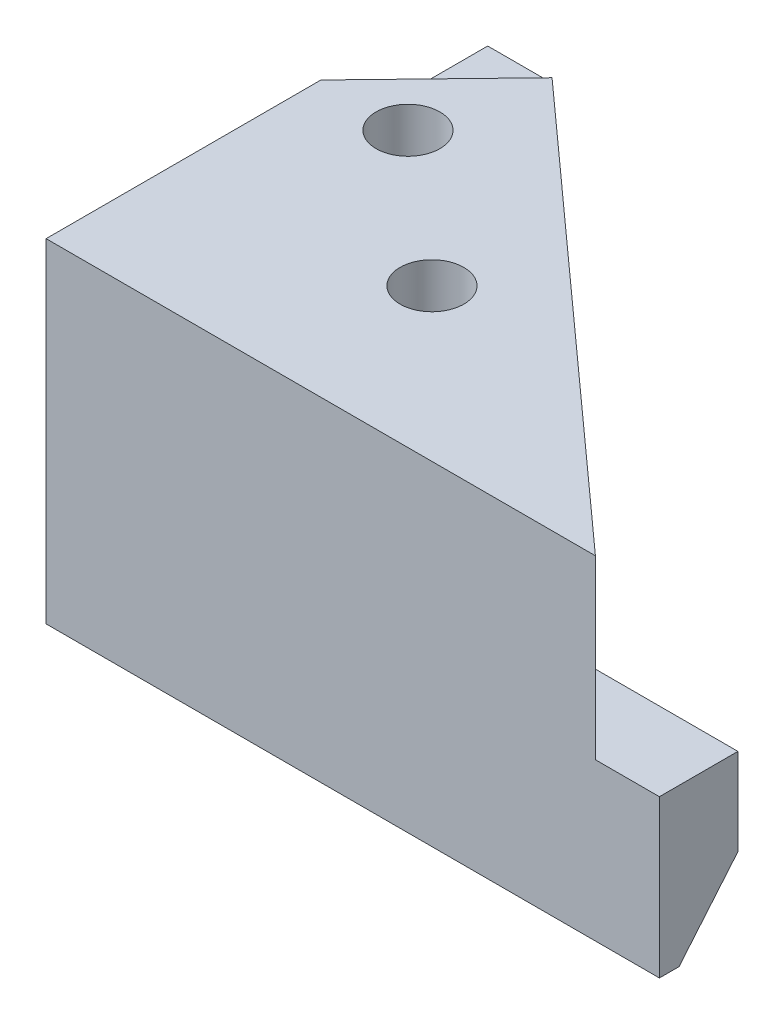
ISO-10303-21;
HEADER;
FILE_DESCRIPTION(('STEP AP214'),'2;1');
FILE_NAME('part.step','',(''),(''),'','','');
FILE_SCHEMA(('AUTOMOTIVE_DESIGN { 1 0 10303 214 1 1 1 1 }'));
ENDSEC;
DATA;
#1=APPLICATION_CONTEXT('core data for automotive mechanical design processes');
#2=APPLICATION_PROTOCOL_DEFINITION('international standard','automotive_design',2000,#1);
#3=PRODUCT_CONTEXT('',#1,'mechanical');
#4=PRODUCT('Part','Part','',(#3));
#5=PRODUCT_RELATED_PRODUCT_CATEGORY('part','',(#4));
#6=PRODUCT_DEFINITION_FORMATION('','',#4);
#7=PRODUCT_DEFINITION_CONTEXT('part definition',#1,'design');
#8=PRODUCT_DEFINITION('design','',#6,#7);
#9=PRODUCT_DEFINITION_SHAPE('','',#8);
#10=(LENGTH_UNIT() NAMED_UNIT(*) SI_UNIT(.MILLI.,.METRE.));
#11=(NAMED_UNIT(*) PLANE_ANGLE_UNIT() SI_UNIT($,.RADIAN.));
#12=(NAMED_UNIT(*) SI_UNIT($,.STERADIAN.) SOLID_ANGLE_UNIT());
#13=UNCERTAINTY_MEASURE_WITH_UNIT(LENGTH_MEASURE(1.E-05),#10,'distance_accuracy_value','');
#14=(GEOMETRIC_REPRESENTATION_CONTEXT(3) GLOBAL_UNCERTAINTY_ASSIGNED_CONTEXT((#13)) GLOBAL_UNIT_ASSIGNED_CONTEXT((#10,
#11,#12)) REPRESENTATION_CONTEXT('',''));
#15=CARTESIAN_POINT('',(0.,0.,0.));
#16=DIRECTION('',(0.,0.,1.));
#17=DIRECTION('',(1.,0.,0.));
#18=AXIS2_PLACEMENT_3D('',#15,#16,#17);
#19=CARTESIAN_POINT('',(0.,36.,0.));
#20=DIRECTION('',(-0.669130606358854,0.,0.743144825477398));
#21=DIRECTION('',(0.743144825477398,0.,0.669130606358854));
#22=AXIS2_PLACEMENT_3D('',#19,#20,#21);
#23=PLANE('',#22);
#24=CARTESIAN_POINT('',(-49.7907033069857,17.,-44.8317506260432));
#25=DIRECTION('',(0.669130606358854,0.,-0.743144825477398));
#26=DIRECTION('',(-0.743144825477398,0.,-0.669130606358854));
#27=AXIS2_PLACEMENT_3D('',#24,#25,#26);
#28=CIRCLE('',#27,6.);
#29=CARTESIAN_POINT('',(-54.2495722598501,17.,-48.8465342641963));
#30=VERTEX_POINT('',#29);
#31=EDGE_CURVE('E312',#30,#30,#28,.T.);
#32=ORIENTED_EDGE('',*,*,#31,.F.);
#33=EDGE_LOOP('',(#32));
#34=FACE_BOUND('',#33,.T.);
#35=DIRECTION('',(0.,-1.,0.));
#36=VECTOR('',#35,1.);
#37=CARTESIAN_POINT('',(-88.8009956275672,266.1095550301,-79.9567756007354));
#38=LINE('',#37,#36);
#39=CARTESIAN_POINT('',(-88.8009956275672,36.,-79.9567756007354));
#40=VERTEX_POINT('',#39);
#41=CARTESIAN_POINT('',(-88.8009956275672,25.,-79.9567756007354));
#42=VERTEX_POINT('',#41);
#43=EDGE_CURVE('E297',#40,#42,#38,.T.);
#44=ORIENTED_EDGE('',*,*,#43,.F.);
#45=DIRECTION('',(-0.743144825477398,0.,-0.669130606358854));
#46=VECTOR('',#45,1.);
#47=CARTESIAN_POINT('',(0.,36.,0.));
#48=LINE('',#47,#46);
#49=CARTESIAN_POINT('',(0.,36.,0.));
#50=VERTEX_POINT('',#49);
#51=EDGE_CURVE('E261',#50,#40,#48,.T.);
#52=ORIENTED_EDGE('',*,*,#51,.F.);
#53=DIRECTION('',(0.,-1.,0.));
#54=VECTOR('',#53,1.);
#55=CARTESIAN_POINT('',(0.,36.,0.));
#56=LINE('',#55,#54);
#57=CARTESIAN_POINT('',(0.,0.,0.));
#58=VERTEX_POINT('',#57);
#59=EDGE_CURVE('E11',#50,#58,#56,.T.);
#60=ORIENTED_EDGE('',*,*,#59,.T.);
#61=DIRECTION('',(-0.743144825477398,0.,-0.669130606358854));
#62=VECTOR('',#61,1.);
#63=CARTESIAN_POINT('',(0.,0.,0.));
#64=LINE('',#63,#62);
#65=CARTESIAN_POINT('',(-17.7698002372673,0.,-16.));
#66=VERTEX_POINT('',#65);
#67=EDGE_CURVE('E262',#58,#66,#64,.T.);
#68=ORIENTED_EDGE('',*,*,#67,.T.);
#69=CARTESIAN_POINT('',(-99.9551263346285,0.,-90.));
#70=VERTEX_POINT('',#69);
#71=EDGE_CURVE('E267',#66,#70,#64,.T.);
#72=ORIENTED_EDGE('',*,*,#71,.T.);
#73=DIRECTION('',(0.,-1.,0.));
#74=VECTOR('',#73,1.);
#75=CARTESIAN_POINT('',(-99.9551263346285,36.,-90.));
#76=LINE('',#75,#74);
#77=CARTESIAN_POINT('',(-99.9551263346285,25.,-90.));
#78=VERTEX_POINT('',#77);
#79=EDGE_CURVE('E47',#78,#70,#76,.T.);
#80=ORIENTED_EDGE('',*,*,#79,.F.);
#81=DIRECTION('',(-0.743144825477398,0.,-0.669130606358854));
#82=VECTOR('',#81,1.);
#83=CARTESIAN_POINT('',(0.,25.,0.));
#84=LINE('',#83,#82);
#85=EDGE_CURVE('E291',#42,#78,#84,.T.);
#86=ORIENTED_EDGE('',*,*,#85,.F.);
#87=EDGE_LOOP('',(#44,#52,#60,#68,#72,#80,#86));
#88=FACE_BOUND('',#87,.T.);
#89=ADVANCED_FACE('F39',(#34,#88),#23,.F.);
#90=CARTESIAN_POINT('',(-99.9551263346285,36.,-90.));
#91=DIRECTION('',(0.,0.,1.));
#92=DIRECTION('',(1.,0.,0.));
#93=AXIS2_PLACEMENT_3D('',#90,#91,#92);
#94=PLANE('',#93);
#95=DIRECTION('',(-1.,0.,0.));
#96=VECTOR('',#95,1.);
#97=CARTESIAN_POINT('',(-99.9551263346285,25.,-90.));
#98=LINE('',#97,#96);
#99=CARTESIAN_POINT('',(-111.955126334629,25.,-90.));
#100=VERTEX_POINT('',#99);
#101=EDGE_CURVE('E278',#78,#100,#98,.T.);
#102=ORIENTED_EDGE('',*,*,#101,.F.);
#103=ORIENTED_EDGE('',*,*,#79,.T.);
#104=DIRECTION('',(-1.,0.,0.));
#105=VECTOR('',#104,1.);
#106=CARTESIAN_POINT('',(-99.9551263346285,0.,-90.));
#107=LINE('',#106,#105);
#108=CARTESIAN_POINT('',(-111.955126334629,0.,-90.));
#109=VERTEX_POINT('',#108);
#110=EDGE_CURVE('E256',#70,#109,#107,.T.);
#111=ORIENTED_EDGE('',*,*,#110,.T.);
#112=DIRECTION('',(0.,-1.,0.));
#113=VECTOR('',#112,1.);
#114=CARTESIAN_POINT('',(-111.955126334629,36.,-90.));
#115=LINE('',#114,#113);
#116=EDGE_CURVE('E241',#100,#109,#115,.T.);
#117=ORIENTED_EDGE('',*,*,#116,.F.);
#118=EDGE_LOOP('',(#102,#103,#111,#117));
#119=FACE_BOUND('',#118,.T.);
#120=ADVANCED_FACE('F239',(#119),#94,.F.);
#121=CARTESIAN_POINT('',(-111.955126334628,36.,0.));
#122=DIRECTION('',(0.,0.,-1.));
#123=DIRECTION('',(-1.,0.,0.));
#124=AXIS2_PLACEMENT_3D('',#121,#122,#123);
#125=PLANE('',#124);
#126=DIRECTION('',(0.,-1.,0.));
#127=VECTOR('',#126,1.);
#128=CARTESIAN_POINT('',(-111.955126334628,36.,0.));
#129=LINE('',#128,#127);
#130=CARTESIAN_POINT('',(-111.955126334628,36.,0.));
#131=VERTEX_POINT('',#130);
#132=CARTESIAN_POINT('',(-111.957563167314,0.,0.));
#133=VERTEX_POINT('',#132);
#134=EDGE_CURVE('E148',#131,#133,#129,.T.);
#135=ORIENTED_EDGE('',*,*,#134,.T.);
#136=DIRECTION('',(0.,-1.,0.));
#137=VECTOR('',#136,1.);
#138=CARTESIAN_POINT('',(-111.96,0.,0.));
#139=LINE('',#138,#137);
#140=CARTESIAN_POINT('',(-111.96,-32.,0.));
#141=VERTEX_POINT('',#140);
#142=EDGE_CURVE('E137',#133,#141,#139,.T.);
#143=ORIENTED_EDGE('',*,*,#142,.T.);
#144=DIRECTION('',(1.,0.,0.));
#145=VECTOR('',#144,1.);
#146=CARTESIAN_POINT('',(-111.96,-32.,0.));
#147=LINE('',#146,#145);
#148=CARTESIAN_POINT('',(13.04,-32.,0.));
#149=VERTEX_POINT('',#148);
#150=EDGE_CURVE('E116',#141,#149,#147,.T.);
#151=ORIENTED_EDGE('',*,*,#150,.T.);
#152=DIRECTION('',(0.,-1.,0.));
#153=VECTOR('',#152,1.);
#154=CARTESIAN_POINT('',(13.04,0.,0.));
#155=LINE('',#154,#153);
#156=CARTESIAN_POINT('',(13.04,0.,0.));
#157=VERTEX_POINT('',#156);
#158=EDGE_CURVE('E180',#157,#149,#155,.T.);
#159=ORIENTED_EDGE('',*,*,#158,.F.);
#160=DIRECTION('',(1.,0.,0.));
#161=VECTOR('',#160,1.);
#162=CARTESIAN_POINT('',(-111.96,0.,0.));
#163=LINE('',#162,#161);
#164=EDGE_CURVE('E165',#58,#157,#163,.T.);
#165=ORIENTED_EDGE('',*,*,#164,.F.);
#166=ORIENTED_EDGE('',*,*,#59,.F.);
#167=DIRECTION('',(1.,0.,0.));
#168=VECTOR('',#167,1.);
#169=CARTESIAN_POINT('',(-111.955126334628,36.,0.));
#170=LINE('',#169,#168);
#171=EDGE_CURVE('E260',#131,#50,#170,.T.);
#172=ORIENTED_EDGE('',*,*,#171,.F.);
#173=EDGE_LOOP('',(#135,#143,#151,#159,#165,#166,#172));
#174=FACE_BOUND('',#173,.T.);
#175=ADVANCED_FACE('F41',(#174),#125,.F.);
#176=CARTESIAN_POINT('',(-111.955126334629,36.,-90.));
#177=DIRECTION('',(1.,0.,0.));
#178=DIRECTION('',(0.,0.,-1.));
#179=AXIS2_PLACEMENT_3D('',#176,#177,#178);
#180=PLANE('',#179);
#181=DIRECTION('',(0.,0.,1.));
#182=VECTOR('',#181,1.);
#183=CARTESIAN_POINT('',(-111.955126334629,36.,-90.));
#184=LINE('',#183,#182);
#185=CARTESIAN_POINT('',(-111.955126334629,36.,-56.));
#186=VERTEX_POINT('',#185);
#187=EDGE_CURVE('E271',#186,#131,#184,.T.);
#188=ORIENTED_EDGE('',*,*,#187,.F.);
#189=DIRECTION('',(0.,-1.,0.));
#190=VECTOR('',#189,1.);
#191=CARTESIAN_POINT('',(-111.955126334629,266.1095550301,-56.));
#192=LINE('',#191,#190);
#193=CARTESIAN_POINT('',(-111.955126334629,25.,-56.));
#194=VERTEX_POINT('',#193);
#195=EDGE_CURVE('E290',#186,#194,#192,.T.);
#196=ORIENTED_EDGE('',*,*,#195,.T.);
#197=DIRECTION('',(0.,0.,1.));
#198=VECTOR('',#197,1.);
#199=CARTESIAN_POINT('',(-111.955126334629,25.,-90.));
#200=LINE('',#199,#198);
#201=EDGE_CURVE('E286',#100,#194,#200,.T.);
#202=ORIENTED_EDGE('',*,*,#201,.F.);
#203=ORIENTED_EDGE('',*,*,#116,.T.);
#204=DIRECTION('',(0.,0.,-1.));
#205=VECTOR('',#204,1.);
#206=CARTESIAN_POINT('',(-111.955126334629,0.,-90.));
#207=LINE('',#206,#205);
#208=CARTESIAN_POINT('',(-111.957313167314,0.,-16.));
#209=VERTEX_POINT('',#208);
#210=EDGE_CURVE('E258',#109,#209,#207,.F.);
#211=ORIENTED_EDGE('',*,*,#210,.T.);
#212=CARTESIAN_POINT('',(-111.955126334628,0.,-16.));
#213=DIRECTION('',(0.,0.,1.));
#214=VECTOR('',#213,1.);
#215=LINE('',#212,#214);
#216=EDGE_CURVE('E133',#209,#133,#215,.T.);
#217=ORIENTED_EDGE('',*,*,#216,.T.);
#218=ORIENTED_EDGE('',*,*,#134,.F.);
#219=EDGE_LOOP('',(#188,#196,#202,#203,#211,#217,#218));
#220=FACE_BOUND('',#219,.T.);
#221=ADVANCED_FACE('F226',(#220),#180,.F.);
#222=CARTESIAN_POINT('',(0.,36.,0.));
#223=DIRECTION('',(0.,-1.,0.));
#224=DIRECTION('',(0.,0.,-1.));
#225=AXIS2_PLACEMENT_3D('',#222,#223,#224);
#226=PLANE('',#225);
#227=CARTESIAN_POINT('',(-64.3185189569977,36.,-31.));
#228=DIRECTION('',(0.,-1.,0.));
#229=DIRECTION('',(0.,0.,-1.));
#230=AXIS2_PLACEMENT_3D('',#227,#228,#229);
#231=CIRCLE('',#230,6.5);
#232=CARTESIAN_POINT('',(-64.3185189569977,36.,-37.5));
#233=VERTEX_POINT('',#232);
#234=EDGE_CURVE('E320',#233,#233,#231,.F.);
#235=ORIENTED_EDGE('',*,*,#234,.F.);
#236=EDGE_LOOP('',(#235));
#237=FACE_BOUND('',#236,.T.);
#238=CARTESIAN_POINT('',(-94.2028213467131,36.,-56.));
#239=DIRECTION('',(0.,-1.,0.));
#240=DIRECTION('',(0.,0.,-1.));
#241=AXIS2_PLACEMENT_3D('',#238,#239,#240);
#242=CIRCLE('',#241,6.5);
#243=CARTESIAN_POINT('',(-94.2028213467131,36.,-62.5));
#244=VERTEX_POINT('',#243);
#245=EDGE_CURVE('E330',#244,#244,#242,.F.);
#246=ORIENTED_EDGE('',*,*,#245,.F.);
#247=EDGE_LOOP('',(#246));
#248=FACE_BOUND('',#247,.T.);
#249=ORIENTED_EDGE('',*,*,#51,.T.);
#250=DIRECTION('',(-0.694958701121631,0.,0.719049653177954));
#251=VECTOR('',#250,1.);
#252=CARTESIAN_POINT('',(-111.955126334629,36.,-56.));
#253=LINE('',#252,#251);
#254=EDGE_CURVE('E288',#40,#186,#253,.T.);
#255=ORIENTED_EDGE('',*,*,#254,.T.);
#256=ORIENTED_EDGE('',*,*,#187,.T.);
#257=ORIENTED_EDGE('',*,*,#171,.T.);
#258=EDGE_LOOP('',(#249,#255,#256,#257));
#259=FACE_BOUND('',#258,.T.);
#260=ADVANCED_FACE('F229',(#237,#248,#259),#226,.F.);
#261=CARTESIAN_POINT('',(0.,0.,0.));
#262=DIRECTION('',(0.,-1.,0.));
#263=DIRECTION('',(0.,0.,-1.));
#264=AXIS2_PLACEMENT_3D('',#261,#262,#263);
#265=PLANE('',#264);
#266=CARTESIAN_POINT('',(-64.3185189569977,0.,-31.));
#267=DIRECTION('',(0.,-1.,0.));
#268=DIRECTION('',(0.,0.,-1.));
#269=AXIS2_PLACEMENT_3D('',#266,#267,#268);
#270=CIRCLE('',#269,6.5);
#271=CARTESIAN_POINT('',(-64.3185189569977,0.,-37.5));
#272=VERTEX_POINT('',#271);
#273=EDGE_CURVE('E321',#272,#272,#270,.T.);
#274=ORIENTED_EDGE('',*,*,#273,.F.);
#275=EDGE_LOOP('',(#274));
#276=FACE_BOUND('',#275,.T.);
#277=CARTESIAN_POINT('',(-94.2028213467131,0.,-56.));
#278=DIRECTION('',(0.,-1.,0.));
#279=DIRECTION('',(0.,0.,-1.));
#280=AXIS2_PLACEMENT_3D('',#277,#278,#279);
#281=CIRCLE('',#280,6.5);
#282=CARTESIAN_POINT('',(-94.2028213467131,0.,-62.5));
#283=VERTEX_POINT('',#282);
#284=EDGE_CURVE('E322',#283,#283,#281,.T.);
#285=ORIENTED_EDGE('',*,*,#284,.F.);
#286=EDGE_LOOP('',(#285));
#287=FACE_BOUND('',#286,.T.);
#288=DIRECTION('',(1.,0.,0.));
#289=VECTOR('',#288,1.);
#290=CARTESIAN_POINT('',(-111.96,0.,-16.));
#291=LINE('',#290,#289);
#292=EDGE_CURVE('E60',#209,#66,#291,.T.);
#293=ORIENTED_EDGE('',*,*,#292,.F.);
#294=ORIENTED_EDGE('',*,*,#210,.F.);
#295=ORIENTED_EDGE('',*,*,#110,.F.);
#296=ORIENTED_EDGE('',*,*,#71,.F.);
#297=EDGE_LOOP('',(#293,#294,#295,#296));
#298=FACE_BOUND('',#297,.T.);
#299=ADVANCED_FACE('F225',(#276,#287,#298),#265,.T.);
#300=CARTESIAN_POINT('',(-111.955126334629,266.1095550301,-56.));
#301=DIRECTION('',(-0.719049653177954,0.,-0.694958701121631));
#302=DIRECTION('',(-0.694958701121631,0.,0.719049653177954));
#303=AXIS2_PLACEMENT_3D('',#300,#301,#302);
#304=PLANE('',#303);
#305=ORIENTED_EDGE('',*,*,#254,.F.);
#306=ORIENTED_EDGE('',*,*,#43,.T.);
#307=DIRECTION('',(-0.694958701121631,0.,0.719049653177954));
#308=VECTOR('',#307,1.);
#309=CARTESIAN_POINT('',(-111.955126334629,25.,-56.));
#310=LINE('',#309,#308);
#311=EDGE_CURVE('E292',#42,#194,#310,.T.);
#312=ORIENTED_EDGE('',*,*,#311,.T.);
#313=ORIENTED_EDGE('',*,*,#195,.F.);
#314=EDGE_LOOP('',(#305,#306,#312,#313));
#315=FACE_BOUND('',#314,.T.);
#316=ADVANCED_FACE('F218',(#315),#304,.T.);
#317=CARTESIAN_POINT('',(0.,25.,0.));
#318=DIRECTION('',(0.,-1.,0.));
#319=DIRECTION('',(0.,0.,-1.));
#320=AXIS2_PLACEMENT_3D('',#317,#318,#319);
#321=PLANE('',#320);
#322=ORIENTED_EDGE('',*,*,#201,.T.);
#323=ORIENTED_EDGE('',*,*,#311,.F.);
#324=ORIENTED_EDGE('',*,*,#85,.T.);
#325=ORIENTED_EDGE('',*,*,#101,.T.);
#326=EDGE_LOOP('',(#322,#323,#324,#325));
#327=FACE_BOUND('',#326,.T.);
#328=ADVANCED_FACE('F209',(#327),#321,.F.);
#329=CARTESIAN_POINT('',(-111.96,0.,0.));
#330=DIRECTION('',(0.,1.,0.));
#331=DIRECTION('',(0.,0.,1.));
#332=AXIS2_PLACEMENT_3D('',#329,#330,#331);
#333=PLANE('',#332);
#334=ORIENTED_EDGE('',*,*,#67,.F.);
#335=ORIENTED_EDGE('',*,*,#164,.T.);
#336=DIRECTION('',(0.,0.,1.));
#337=VECTOR('',#336,1.);
#338=CARTESIAN_POINT('',(13.04,0.,0.));
#339=LINE('',#338,#337);
#340=CARTESIAN_POINT('',(13.04,0.,-16.));
#341=VERTEX_POINT('',#340);
#342=EDGE_CURVE('E150',#341,#157,#339,.T.);
#343=ORIENTED_EDGE('',*,*,#342,.F.);
#344=EDGE_CURVE('E158',#66,#341,#291,.T.);
#345=ORIENTED_EDGE('',*,*,#344,.F.);
#346=EDGE_LOOP('',(#334,#335,#343,#345));
#347=FACE_BOUND('',#346,.T.);
#348=ADVANCED_FACE('F206',(#347),#333,.T.);
#349=CARTESIAN_POINT('',(-111.96,0.,-16.));
#350=DIRECTION('',(0.,0.,-1.));
#351=DIRECTION('',(0.,1.,0.));
#352=AXIS2_PLACEMENT_3D('',#349,#350,#351);
#353=PLANE('',#352);
#354=DIRECTION('',(0.,1.,0.));
#355=VECTOR('',#354,1.);
#356=CARTESIAN_POINT('',(13.04,0.,-16.));
#357=LINE('',#356,#355);
#358=CARTESIAN_POINT('',(13.04,-17.6989568888696,-16.));
#359=VERTEX_POINT('',#358);
#360=EDGE_CURVE('E147',#359,#341,#357,.T.);
#361=ORIENTED_EDGE('',*,*,#360,.F.);
#362=DIRECTION('',(1.,0.,0.));
#363=VECTOR('',#362,1.);
#364=CARTESIAN_POINT('',(-111.96,-17.6989568888696,-16.));
#365=LINE('',#364,#363);
#366=CARTESIAN_POINT('',(-111.96,-17.6989568888696,-16.));
#367=VERTEX_POINT('',#366);
#368=EDGE_CURVE('E161',#367,#359,#365,.T.);
#369=ORIENTED_EDGE('',*,*,#368,.F.);
#370=DIRECTION('',(0.,1.,0.));
#371=VECTOR('',#370,1.);
#372=CARTESIAN_POINT('',(-111.96,0.,-16.));
#373=LINE('',#372,#371);
#374=EDGE_CURVE('E169',#367,#209,#373,.T.);
#375=ORIENTED_EDGE('',*,*,#374,.T.);
#376=ORIENTED_EDGE('',*,*,#292,.T.);
#377=ORIENTED_EDGE('',*,*,#344,.T.);
#378=EDGE_LOOP('',(#361,#369,#375,#376,#377));
#379=FACE_BOUND('',#378,.T.);
#380=ADVANCED_FACE('F207',(#379),#353,.T.);
#381=CARTESIAN_POINT('',(-111.96,-17.6989568888696,-16.));
#382=DIRECTION('',(0.,-0.642787609686543,-0.766044443118975));
#383=DIRECTION('',(0.,0.766044443118975,-0.642787609686543));
#384=AXIS2_PLACEMENT_3D('',#381,#382,#383);
#385=PLANE('',#384);
#386=DIRECTION('',(0.,0.766044443118975,-0.642787609686543));
#387=VECTOR('',#386,1.);
#388=CARTESIAN_POINT('',(13.04,-17.6989568888696,-16.));
#389=LINE('',#388,#387);
#390=CARTESIAN_POINT('',(13.04,-32.,-4.));
#391=VERTEX_POINT('',#390);
#392=EDGE_CURVE('E182',#391,#359,#389,.T.);
#393=ORIENTED_EDGE('',*,*,#392,.F.);
#394=DIRECTION('',(1.,0.,0.));
#395=VECTOR('',#394,1.);
#396=CARTESIAN_POINT('',(-111.96,-32.,-4.));
#397=LINE('',#396,#395);
#398=CARTESIAN_POINT('',(-111.96,-32.,-4.));
#399=VERTEX_POINT('',#398);
#400=EDGE_CURVE('E128',#399,#391,#397,.T.);
#401=ORIENTED_EDGE('',*,*,#400,.F.);
#402=DIRECTION('',(0.,0.766044443118975,-0.642787609686543));
#403=VECTOR('',#402,1.);
#404=CARTESIAN_POINT('',(-111.96,-17.6989568888696,-16.));
#405=LINE('',#404,#403);
#406=EDGE_CURVE('E143',#399,#367,#405,.T.);
#407=ORIENTED_EDGE('',*,*,#406,.T.);
#408=ORIENTED_EDGE('',*,*,#368,.T.);
#409=EDGE_LOOP('',(#393,#401,#407,#408));
#410=FACE_BOUND('',#409,.T.);
#411=ADVANCED_FACE('F212',(#410),#385,.T.);
#412=CARTESIAN_POINT('',(-111.96,-32.,0.));
#413=DIRECTION('',(0.,-1.,0.));
#414=DIRECTION('',(0.,0.,-1.));
#415=AXIS2_PLACEMENT_3D('',#412,#413,#414);
#416=PLANE('',#415);
#417=DIRECTION('',(0.,0.,-1.));
#418=VECTOR('',#417,1.);
#419=CARTESIAN_POINT('',(13.04,-32.,0.));
#420=LINE('',#419,#418);
#421=EDGE_CURVE('E124',#149,#391,#420,.T.);
#422=ORIENTED_EDGE('',*,*,#421,.F.);
#423=ORIENTED_EDGE('',*,*,#150,.F.);
#424=DIRECTION('',(0.,0.,-1.));
#425=VECTOR('',#424,1.);
#426=CARTESIAN_POINT('',(-111.96,-32.,0.));
#427=LINE('',#426,#425);
#428=EDGE_CURVE('E122',#141,#399,#427,.T.);
#429=ORIENTED_EDGE('',*,*,#428,.T.);
#430=ORIENTED_EDGE('',*,*,#400,.T.);
#431=EDGE_LOOP('',(#422,#423,#429,#430));
#432=FACE_BOUND('',#431,.T.);
#433=ADVANCED_FACE('F125',(#432),#416,.T.);
#434=CARTESIAN_POINT('',(-111.96,0.,0.));
#435=DIRECTION('',(1.,0.,0.));
#436=DIRECTION('',(0.,0.,-1.));
#437=AXIS2_PLACEMENT_3D('',#434,#435,#436);
#438=PLANE('',#437);
#439=ORIENTED_EDGE('',*,*,#142,.F.);
#440=ORIENTED_EDGE('',*,*,#216,.F.);
#441=ORIENTED_EDGE('',*,*,#374,.F.);
#442=ORIENTED_EDGE('',*,*,#406,.F.);
#443=ORIENTED_EDGE('',*,*,#428,.F.);
#444=EDGE_LOOP('',(#439,#440,#441,#442,#443));
#445=FACE_BOUND('',#444,.T.);
#446=ADVANCED_FACE('F136',(#445),#438,.F.);
#447=CARTESIAN_POINT('',(13.04,0.,0.));
#448=DIRECTION('',(1.,0.,0.));
#449=DIRECTION('',(0.,0.,-1.));
#450=AXIS2_PLACEMENT_3D('',#447,#448,#449);
#451=PLANE('',#450);
#452=ORIENTED_EDGE('',*,*,#158,.T.);
#453=ORIENTED_EDGE('',*,*,#421,.T.);
#454=ORIENTED_EDGE('',*,*,#392,.T.);
#455=ORIENTED_EDGE('',*,*,#360,.T.);
#456=ORIENTED_EDGE('',*,*,#342,.T.);
#457=EDGE_LOOP('',(#452,#453,#454,#455,#456));
#458=FACE_BOUND('',#457,.T.);
#459=ADVANCED_FACE('F199',(#458),#451,.T.);
#460=CARTESIAN_POINT('',(-57.1511399769331,17.,-36.6571575457918));
#461=DIRECTION('',(0.669130606358854,0.,-0.743144825477398));
#462=DIRECTION('',(-0.743144825477398,0.,-0.669130606358854));
#463=AXIS2_PLACEMENT_3D('',#460,#461,#462);
#464=CYLINDRICAL_SURFACE('',#463,6.);
#465=CARTESIAN_POINT('',(-57.1511399769331,17.,-36.6571575457918));
#466=DIRECTION('',(0.669130606358854,0.,-0.743144825477398));
#467=DIRECTION('',(-0.743144825477398,0.,-0.669130606358854));
#468=AXIS2_PLACEMENT_3D('',#465,#466,#467);
#469=CIRCLE('',#468,6.);
#470=CARTESIAN_POINT('',(-61.6100089297975,17.,-40.671941183945));
#471=VERTEX_POINT('',#470);
#472=EDGE_CURVE('E178',#471,#471,#469,.T.);
#473=ORIENTED_EDGE('',*,*,#472,.F.);
#474=EDGE_LOOP('',(#473));
#475=FACE_BOUND('',#474,.T.);
#476=ORIENTED_EDGE('',*,*,#31,.T.);
#477=EDGE_LOOP('',(#476));
#478=FACE_BOUND('',#477,.T.);
#479=ADVANCED_FACE('F203',(#475,#478),#464,.F.);
#480=CARTESIAN_POINT('',(-57.1511399769331,17.,-36.6571575457918));
#481=DIRECTION('',(0.669130606358854,0.,-0.743144825477398));
#482=DIRECTION('',(-0.743144825477398,0.,-0.669130606358854));
#483=AXIS2_PLACEMENT_3D('',#480,#481,#482);
#484=PLANE('',#483);
#485=ORIENTED_EDGE('',*,*,#472,.T.);
#486=EDGE_LOOP('',(#485));
#487=FACE_BOUND('',#486,.T.);
#488=ADVANCED_FACE('F341',(#487),#484,.T.);
#489=CARTESIAN_POINT('',(-94.2028213467131,36.001025,-56.));
#490=DIRECTION('',(0.,-1.,0.));
#491=DIRECTION('',(0.,0.,-1.));
#492=AXIS2_PLACEMENT_3D('',#489,#490,#491);
#493=CYLINDRICAL_SURFACE('',#492,6.5);
#494=CARTESIAN_POINT('',(-94.2028213467131,0.,-62.5));
#495=CARTESIAN_POINT('',(-94.2028213467131,0.375,-62.5));
#496=CARTESIAN_POINT('',(-94.2028213467131,0.750000000000001,-62.5));
#497=CARTESIAN_POINT('',(-94.2028213467131,1.5,-62.5));
#498=CARTESIAN_POINT('',(-94.2028213467131,1.875,-62.5));
#499=CARTESIAN_POINT('',(-94.2028213467131,2.625,-62.5));
#500=CARTESIAN_POINT('',(-94.2028213467131,3.,-62.5));
#501=CARTESIAN_POINT('',(-94.2028213467131,3.75,-62.5));
#502=CARTESIAN_POINT('',(-94.2028213467131,4.125,-62.5));
#503=CARTESIAN_POINT('',(-94.2028213467131,4.875,-62.5));
#504=CARTESIAN_POINT('',(-94.2028213467131,5.25,-62.5));
#505=CARTESIAN_POINT('',(-94.2028213467131,6.,-62.5));
#506=CARTESIAN_POINT('',(-94.2028213467131,6.375,-62.5));
#507=CARTESIAN_POINT('',(-94.2028213467131,7.125,-62.5));
#508=CARTESIAN_POINT('',(-94.2028213467131,7.5,-62.5));
#509=CARTESIAN_POINT('',(-94.2028213467131,8.25,-62.5));
#510=CARTESIAN_POINT('',(-94.2028213467131,8.625,-62.5));
#511=CARTESIAN_POINT('',(-94.2028213467131,9.375,-62.5));
#512=CARTESIAN_POINT('',(-94.2028213467131,9.75,-62.5));
#513=CARTESIAN_POINT('',(-94.2028213467131,10.5,-62.5));
#514=CARTESIAN_POINT('',(-94.2028213467131,10.875,-62.5));
#515=CARTESIAN_POINT('',(-94.2028213467131,11.625,-62.5));
#516=CARTESIAN_POINT('',(-94.2028213467131,12.,-62.5));
#517=CARTESIAN_POINT('',(-94.2028213467131,12.75,-62.5));
#518=CARTESIAN_POINT('',(-94.2028213467131,13.125,-62.5));
#519=CARTESIAN_POINT('',(-94.2028213467131,13.875,-62.5));
#520=CARTESIAN_POINT('',(-94.2028213467131,14.25,-62.5));
#521=CARTESIAN_POINT('',(-94.2028213467131,15.,-62.5));
#522=CARTESIAN_POINT('',(-94.2028213467131,15.375,-62.5));
#523=CARTESIAN_POINT('',(-94.2028213467131,16.125,-62.5));
#524=CARTESIAN_POINT('',(-94.2028213467131,16.5,-62.5));
#525=CARTESIAN_POINT('',(-94.2028213467131,17.25,-62.5));
#526=CARTESIAN_POINT('',(-94.2028213467131,17.625,-62.5));
#527=CARTESIAN_POINT('',(-94.2028213467131,18.375,-62.5));
#528=CARTESIAN_POINT('',(-94.2028213467131,18.75,-62.5));
#529=CARTESIAN_POINT('',(-94.2028213467131,19.5,-62.5));
#530=CARTESIAN_POINT('',(-94.2028213467131,19.875,-62.5));
#531=CARTESIAN_POINT('',(-94.2028213467131,20.625,-62.5));
#532=CARTESIAN_POINT('',(-94.2028213467131,21.,-62.5));
#533=CARTESIAN_POINT('',(-94.2028213467131,21.75,-62.5));
#534=CARTESIAN_POINT('',(-94.2028213467131,22.125,-62.5));
#535=CARTESIAN_POINT('',(-94.2028213467131,22.875,-62.5));
#536=CARTESIAN_POINT('',(-94.2028213467131,23.25,-62.5));
#537=CARTESIAN_POINT('',(-94.2028213467131,24.,-62.5));
#538=CARTESIAN_POINT('',(-94.2028213467131,24.375,-62.5));
#539=CARTESIAN_POINT('',(-94.2028213467131,25.125,-62.5));
#540=CARTESIAN_POINT('',(-94.2028213467131,25.5,-62.5));
#541=CARTESIAN_POINT('',(-94.2028213467131,26.25,-62.5));
#542=CARTESIAN_POINT('',(-94.2028213467131,26.625,-62.5));
#543=CARTESIAN_POINT('',(-94.2028213467131,27.375,-62.5));
#544=CARTESIAN_POINT('',(-94.2028213467131,27.75,-62.5));
#545=CARTESIAN_POINT('',(-94.2028213467131,28.5,-62.5));
#546=CARTESIAN_POINT('',(-94.2028213467131,28.875,-62.5));
#547=CARTESIAN_POINT('',(-94.2028213467131,29.625,-62.5));
#548=CARTESIAN_POINT('',(-94.2028213467131,30.,-62.5));
#549=CARTESIAN_POINT('',(-94.2028213467131,30.75,-62.5));
#550=CARTESIAN_POINT('',(-94.2028213467131,31.125,-62.5));
#551=CARTESIAN_POINT('',(-94.2028213467131,31.875,-62.5));
#552=CARTESIAN_POINT('',(-94.2028213467131,32.25,-62.5));
#553=CARTESIAN_POINT('',(-94.2028213467131,33.,-62.5));
#554=CARTESIAN_POINT('',(-94.2028213467131,33.375,-62.5));
#555=CARTESIAN_POINT('',(-94.2028213467131,34.125,-62.5));
#556=CARTESIAN_POINT('',(-94.2028213467131,34.5,-62.5));
#557=CARTESIAN_POINT('',(-94.2028213467131,35.25,-62.5));
#558=CARTESIAN_POINT('',(-94.2028213467131,35.625,-62.5));
#559=CARTESIAN_POINT('',(-94.2028213467131,36.,-62.5));
#560=B_SPLINE_CURVE_WITH_KNOTS('',3,(#494,#495,#496,#497,#498,#499,#500,#501,#502,#503,#504,
#505,#506,#507,#508,#509,#510,#511,#512,#513,#514,#515,#516,#517,#518,#519,#520,#521,#522,#523,
#524,#525,#526,#527,#528,#529,#530,#531,#532,#533,#534,#535,#536,#537,#538,#539,#540,#541,#542,
#543,#544,#545,#546,#547,#548,#549,#550,#551,#552,#553,#554,#555,#556,#557,#558,#559),
.UNSPECIFIED.,.F.,.F.,(4,2,2,2,2,2,2,2,2,2,2,2,2,2,2,2,2,2,2,2,2,2,2,2,2,2,2,2,2,2,2,2,4),(0.,
1.125,2.25,3.375,4.5,5.625,6.75,7.875,9.,10.125,11.25,12.375,13.5,14.625,15.75,16.875,18.,
19.125,20.25,21.375,22.5,23.625,24.75,25.875,27.,28.125,29.25,30.375,31.5,32.625,33.75,34.875,
36.),.UNSPECIFIED.);
#561=EDGE_CURVE('BSEAM337',#283,#244,#560,.T.);
#562=ORIENTED_EDGE('',*,*,#284,.T.);
#563=ORIENTED_EDGE('',*,*,#245,.T.);
#564=ORIENTED_EDGE('',*,*,#561,.T.);
#565=ORIENTED_EDGE('',*,*,#561,.F.);
#566=EDGE_LOOP('',(#562,#564,#563,#565));
#567=FACE_BOUND('',#566,.T.);
#568=ADVANCED_FACE('F337',(#567),#493,.F.);
#569=CARTESIAN_POINT('',(-64.3185189569977,36.001025,-31.));
#570=DIRECTION('',(0.,-1.,0.));
#571=DIRECTION('',(0.,0.,-1.));
#572=AXIS2_PLACEMENT_3D('',#569,#570,#571);
#573=CYLINDRICAL_SURFACE('',#572,6.5);
#574=CARTESIAN_POINT('',(-64.3185189569977,0.,-37.5));
#575=CARTESIAN_POINT('',(-64.3185189569977,0.375,-37.5));
#576=CARTESIAN_POINT('',(-64.3185189569977,0.750000000000001,-37.5));
#577=CARTESIAN_POINT('',(-64.3185189569977,1.5,-37.5));
#578=CARTESIAN_POINT('',(-64.3185189569977,1.875,-37.5));
#579=CARTESIAN_POINT('',(-64.3185189569977,2.625,-37.5));
#580=CARTESIAN_POINT('',(-64.3185189569977,3.,-37.5));
#581=CARTESIAN_POINT('',(-64.3185189569977,3.75,-37.5));
#582=CARTESIAN_POINT('',(-64.3185189569977,4.125,-37.5));
#583=CARTESIAN_POINT('',(-64.3185189569977,4.875,-37.5));
#584=CARTESIAN_POINT('',(-64.3185189569977,5.25,-37.5));
#585=CARTESIAN_POINT('',(-64.3185189569977,6.,-37.5));
#586=CARTESIAN_POINT('',(-64.3185189569977,6.375,-37.5));
#587=CARTESIAN_POINT('',(-64.3185189569977,7.125,-37.5));
#588=CARTESIAN_POINT('',(-64.3185189569977,7.5,-37.5));
#589=CARTESIAN_POINT('',(-64.3185189569977,8.25,-37.5));
#590=CARTESIAN_POINT('',(-64.3185189569977,8.625,-37.5));
#591=CARTESIAN_POINT('',(-64.3185189569977,9.375,-37.5));
#592=CARTESIAN_POINT('',(-64.3185189569977,9.75,-37.5));
#593=CARTESIAN_POINT('',(-64.3185189569977,10.5,-37.5));
#594=CARTESIAN_POINT('',(-64.3185189569977,10.875,-37.5));
#595=CARTESIAN_POINT('',(-64.3185189569977,11.625,-37.5));
#596=CARTESIAN_POINT('',(-64.3185189569977,12.,-37.5));
#597=CARTESIAN_POINT('',(-64.3185189569977,12.75,-37.5));
#598=CARTESIAN_POINT('',(-64.3185189569977,13.125,-37.5));
#599=CARTESIAN_POINT('',(-64.3185189569977,13.875,-37.5));
#600=CARTESIAN_POINT('',(-64.3185189569977,14.25,-37.5));
#601=CARTESIAN_POINT('',(-64.3185189569977,15.,-37.5));
#602=CARTESIAN_POINT('',(-64.3185189569977,15.375,-37.5));
#603=CARTESIAN_POINT('',(-64.3185189569977,16.125,-37.5));
#604=CARTESIAN_POINT('',(-64.3185189569977,16.5,-37.5));
#605=CARTESIAN_POINT('',(-64.3185189569977,17.25,-37.5));
#606=CARTESIAN_POINT('',(-64.3185189569977,17.625,-37.5));
#607=CARTESIAN_POINT('',(-64.3185189569977,18.375,-37.5));
#608=CARTESIAN_POINT('',(-64.3185189569977,18.75,-37.5));
#609=CARTESIAN_POINT('',(-64.3185189569977,19.5,-37.5));
#610=CARTESIAN_POINT('',(-64.3185189569977,19.875,-37.5));
#611=CARTESIAN_POINT('',(-64.3185189569977,20.625,-37.5));
#612=CARTESIAN_POINT('',(-64.3185189569977,21.,-37.5));
#613=CARTESIAN_POINT('',(-64.3185189569977,21.75,-37.5));
#614=CARTESIAN_POINT('',(-64.3185189569977,22.125,-37.5));
#615=CARTESIAN_POINT('',(-64.3185189569977,22.875,-37.5));
#616=CARTESIAN_POINT('',(-64.3185189569977,23.25,-37.5));
#617=CARTESIAN_POINT('',(-64.3185189569977,24.,-37.5));
#618=CARTESIAN_POINT('',(-64.3185189569977,24.375,-37.5));
#619=CARTESIAN_POINT('',(-64.3185189569977,25.125,-37.5));
#620=CARTESIAN_POINT('',(-64.3185189569977,25.5,-37.5));
#621=CARTESIAN_POINT('',(-64.3185189569977,26.25,-37.5));
#622=CARTESIAN_POINT('',(-64.3185189569977,26.625,-37.5));
#623=CARTESIAN_POINT('',(-64.3185189569977,27.375,-37.5));
#624=CARTESIAN_POINT('',(-64.3185189569977,27.75,-37.5));
#625=CARTESIAN_POINT('',(-64.3185189569977,28.5,-37.5));
#626=CARTESIAN_POINT('',(-64.3185189569977,28.875,-37.5));
#627=CARTESIAN_POINT('',(-64.3185189569977,29.625,-37.5));
#628=CARTESIAN_POINT('',(-64.3185189569977,30.,-37.5));
#629=CARTESIAN_POINT('',(-64.3185189569977,30.75,-37.5));
#630=CARTESIAN_POINT('',(-64.3185189569977,31.125,-37.5));
#631=CARTESIAN_POINT('',(-64.3185189569977,31.875,-37.5));
#632=CARTESIAN_POINT('',(-64.3185189569977,32.25,-37.5));
#633=CARTESIAN_POINT('',(-64.3185189569977,33.,-37.5));
#634=CARTESIAN_POINT('',(-64.3185189569977,33.375,-37.5));
#635=CARTESIAN_POINT('',(-64.3185189569977,34.125,-37.5));
#636=CARTESIAN_POINT('',(-64.3185189569977,34.5,-37.5));
#637=CARTESIAN_POINT('',(-64.3185189569977,35.25,-37.5));
#638=CARTESIAN_POINT('',(-64.3185189569977,35.625,-37.5));
#639=CARTESIAN_POINT('',(-64.3185189569977,36.,-37.5));
#640=B_SPLINE_CURVE_WITH_KNOTS('',3,(#574,#575,#576,#577,#578,#579,#580,#581,#582,#583,#584,
#585,#586,#587,#588,#589,#590,#591,#592,#593,#594,#595,#596,#597,#598,#599,#600,#601,#602,#603,
#604,#605,#606,#607,#608,#609,#610,#611,#612,#613,#614,#615,#616,#617,#618,#619,#620,#621,#622,
#623,#624,#625,#626,#627,#628,#629,#630,#631,#632,#633,#634,#635,#636,#637,#638,#639),
.UNSPECIFIED.,.F.,.F.,(4,2,2,2,2,2,2,2,2,2,2,2,2,2,2,2,2,2,2,2,2,2,2,2,2,2,2,2,2,2,2,2,4),(0.,
1.125,2.25,3.375,4.5,5.625,6.75,7.875,9.,10.125,11.25,12.375,13.5,14.625,15.75,16.875,18.,
19.125,20.25,21.375,22.5,23.625,24.75,25.875,27.,28.125,29.25,30.375,31.5,32.625,33.75,34.875,
36.),.UNSPECIFIED.);
#641=EDGE_CURVE('BSEAM334',#272,#233,#640,.T.);
#642=ORIENTED_EDGE('',*,*,#273,.T.);
#643=ORIENTED_EDGE('',*,*,#234,.T.);
#644=ORIENTED_EDGE('',*,*,#641,.T.);
#645=ORIENTED_EDGE('',*,*,#641,.F.);
#646=EDGE_LOOP('',(#642,#644,#643,#645));
#647=FACE_BOUND('',#646,.T.);
#648=ADVANCED_FACE('F334',(#647),#573,.F.);
#649=CLOSED_SHELL('',(#89,#120,#175,#221,#260,#299,#316,#328,#348,#380,#411,#433,#446,#459,#479,
#488,#568,#648));
#650=MANIFOLD_SOLID_BREP('B2',#649);
#651=ADVANCED_BREP_SHAPE_REPRESENTATION('',(#18,#650),#14);
#652=SHAPE_DEFINITION_REPRESENTATION(#9,#651);
ENDSEC;
END-ISO-10303-21;
